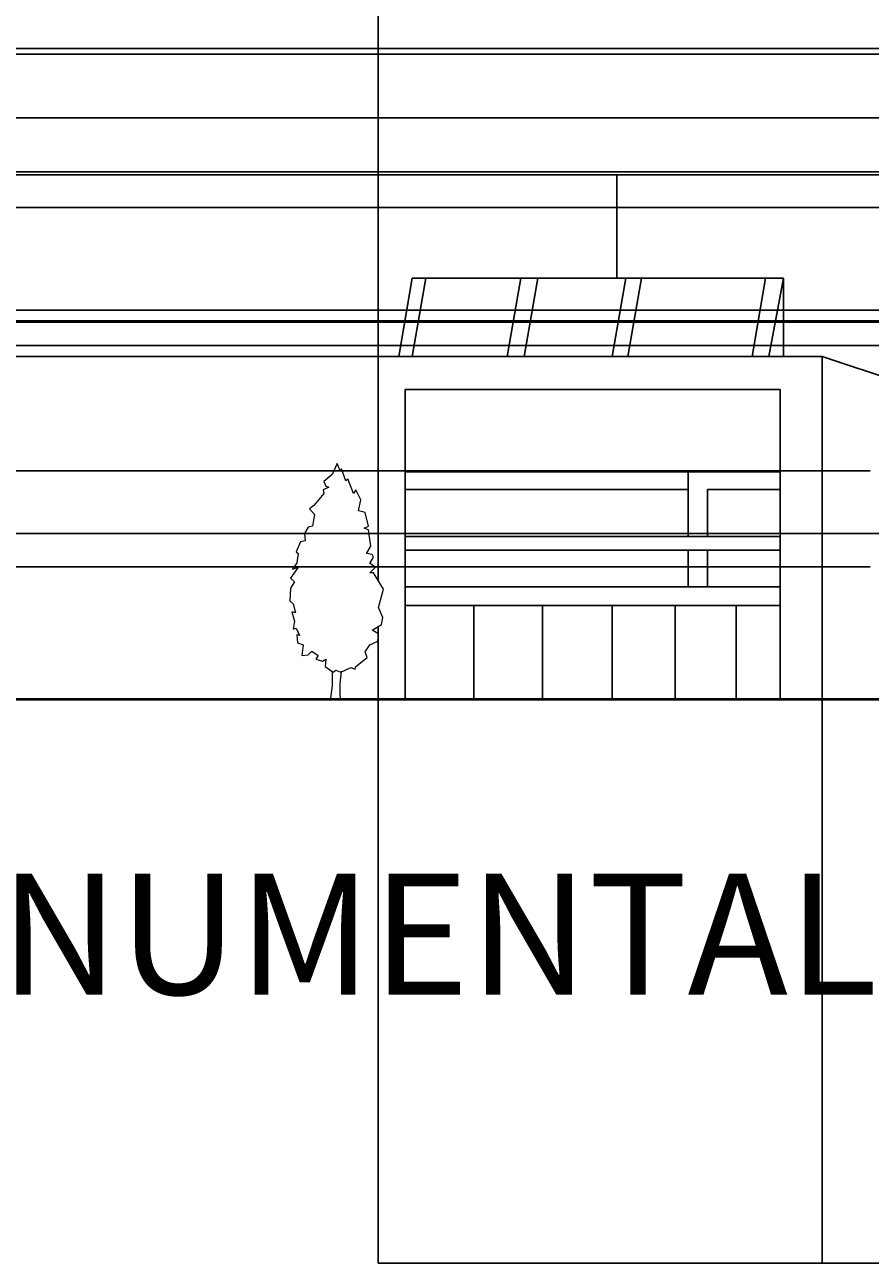
# Model space of a CAD drawing. Units: inches. Extents: x -32109 to 33221, y -19197 to 7608.
# Tile 8 of 25: x -20585 to -15627, y -5430 to 1836. Entities that reach past the tile are written whole.
import ezdxf

# ---------------------------------------------------------------- set-up
doc = ezdxf.new("R2010")
doc.units = ezdxf.units.IN
doc.header["$MEASUREMENT"] = 0
for name, color, linetype, lineweight in [('A-ANNO-DIMS', 2, 'Continuous', 18), ('A-ANNO-TEXT', 7, 'Continuous', 25), ('A-ELEV', 7, 'Continuous', 25), ('L-PLNT', 3, 'Continuous', 13)]:
    doc.layers.add(name, color=color, linetype=linetype, lineweight=lineweight)
doc.styles.get("Standard").update_dxf_attribs({"font": 'arial.ttf'})
doc.dimstyles.get("Standard").update_dxf_attribs({"dimtxt": 0.18, "dimasz": 0.18, "dimexe": 0.18, "dimexo": 0.0625, "dimgap": 0.09, "dimtad": 0, "dimtih": 1, "dimtoh": 1, "dimdec": 4, "dimzin": 0, "dimdsep": 46, "dimtxsty": 'Standard', "dimcen": 0.09, "dimadec": 0, "dimazin": 0, "dimtfac": 1, "dimtdec": 4, "dimtofl": 0, "dimtmove": 0, "dimatfit": 3, "dimfxl": 1, "dimtolj": 1, "dimtzin": 0, "dimarcsym": 0})

# ---------------------------------------------------------------- blocks, each defined once
blk = doc.blocks.new('*U2')
blk.add_lwpolyline([(-2.75400000000036, 191.699), (-6.7800000000002, 182.8509999999996), (-13.68200000000024, 176.9529999999995), (-11.95600000000013, 173.2659999999996), (-9.655999999999949, 172.529), (-14.25700000000006, 170.317), (-13.68200000000024, 167.3679999999999), (-21.73300000000017, 157.7829999999999), (-25.1840000000002, 154.8340000000003), (-21.15800000000036, 150.4099999999998), (-21.73300000000017, 147.4609999999998), (-22.88400000000001, 140.8249999999998), (-26.33400000000029, 140.087), (-29.21000000000004, 134.9259999999995), (-28.63499999999977, 129.0279999999998), (-32.66100000000006, 128.2909999999997), (-36.11099999999988, 120.1799999999998), (-34.38599999999997, 118.7059999999997), (-35.53600000000006, 111.3329999999996), (-38.98700000000008, 106.1709999999998), (-34.38599999999997, 107.6459999999997), (-40.71199999999999, 98.79799999999977), (-37.26099999999997, 95.8489999999997), (-40.71199999999999, 90.68799999999965), (-41.28700000000026, 80.36599999999999), (-38.41200000000026, 78.154), (-36.68600000000015, 70.78099999999995), (-39.5619999999999, 71.51799999999957), (-37.26099999999997, 64.14499999999998), (-38.41200000000026, 57.50899999999956), (-36.11099999999988, 58.24699999999984), (-33.23599999999988, 52.3479999999995), (-35.53600000000006, 53.08599999999978), (-34.96100000000024, 46.44999999999981), (-30.36000000000013, 44.9749999999999), (-31.50999999999977, 36.1279999999997), (-26.33400000000029, 36.86499999999978), (-23.45900000000029, 39.81399999999985), (-18.28300000000036, 36.1279999999997), (-20.00800000000027, 33.17799999999988), (-14.83199999999988, 31.70399999999972), (-11.95600000000013, 33.17799999999988), (-12.53099999999995, 27.27999999999975), (-6.204999999999927, 22.85599999999977), (-3.9050000000002, 24.33099999999968), (0.1209999999996398, 22.85599999999977), (8.172999999999774, 26.54299999999967), (11.62399999999979, 25.06799999999976), (12.19900000000007, 27.27999999999975), (21.40000000000009, 34.6529999999998), (19.67500000000018, 39.07699999999977), (23.70099999999957, 44.9749999999999), (30.02700000000004, 47.92399999999997), (30.60199999999986, 53.82299999999986), (25.42599999999993, 56.77199999999993), (32.90299999999979, 61.19599999999991), (34.05299999999988, 67.0939999999996), (30.60199999999986, 75.20499999999993), (34.6279999999997, 89.95100000000002), (26.57599999999957, 103.2219999999997), (23.70099999999957, 103.2219999999997), (28.30199999999968, 107.6459999999997), (23.70099999999957, 110.5949999999998), (26.57599999999957, 115.7559999999994), (25.42599999999993, 117.9679999999998), (20.82499999999982, 118.7059999999997), (24.27599999999984, 124.6040000000002), (22.55099999999993, 137.8759999999997), (19.09999999999991, 139.3499999999999), (22.55099999999993, 140.8249999999998), (19.67500000000018, 151.884), (14.49899999999979, 153.3589999999999), (16.22400000000016, 162.2069999999999), (12.19900000000007, 170.317), (10.47299999999995, 167.3679999999999), (5.871999999999843, 179.1649999999999), (4.146999999999934, 177.69), (0.6959999999999127, 187.2749999999996), (-0.4540000000001783, 185.7999999999997)], close=True)
for points in [[(-6.813000000000101, 23.66899999999987), (-6.813000000000101, 11.66899999999987), (-8.626999999999953, 0)], [(0.3869999999997162, 23.66899999999987), (-0.5760000000000219, 13.27099999999973), (-0.5760000000000219, 3.685999999999694), (0, 0)]]:
    blk.add_lwpolyline(points)
blk = doc.blocks.new('*D10')
at = {"layer": 'A-ANNO-DIMS', "color": 0, "lineweight": -2, "transparency": 16777216}
for p, q in [((-18512.646816, -110.179138), (-18512.646816, 5772.015489000001)), ((-18512.466816, 5771.835489), (-202.0927503703958, 5771.835489)), ((18109.136745, 5771.835489), (-201.2373206296045, 5771.835489)), ((18109.316745, -101.537382), (18109.316745, 5772.015489000001))]:
    blk.add_line(p, q, dxfattribs=at)
at = {"layer": 'A-ANNO-DIMS', "color": 0, "transparency": 16777216}
for points in [[(-18512.466816, 5771.865488999999), (-18512.466816, 5771.805489000001), (-18512.646816, 5771.835489)], [(18109.136745, 5771.865488999999), (18109.136745, 5771.805489000001), (18109.316745, 5771.835489)]]:
    blk.add_solid(points, dxfattribs=at)
at = {"layer": 'Defpoints', "color": 0, "transparency": 16777216}
for p in [(18109.316745, 5771.835489), (-18512.646816, -110.241638), (18109.316745, -101.599882)]:
    blk.add_point(p, dxfattribs=at)
at = {"layer": 'A-ANNO-DIMS', "color": 0, "transparency": 16777216, "insert": (-201.6650355000002, 5771.835489), "char_height": 0.18, "attachment_point": 5}
blk.add_mtext('\\A1;36622', dxfattribs=at)
blk = doc.blocks.new('*D11')
at = {"layer": 'A-ANNO-DIMS', "color": 0, "lineweight": -2, "transparency": 16777216}
for p, q in [((14509.612941, 1705.161904000001), (25710.64858400003, 1705.161904000003)), ((25710.46858400003, 1704.981904000003), (25710.46858400003, -209.6323674706641)), ((25710.46858400003, -2124.610567999994), (25710.46858400003, -209.9962965293272)), ((-18512.58431600001, -2124.790568000001), (25710.64858400003, -2124.790567999994))]:
    blk.add_line(p, q, dxfattribs=at)
at = {"layer": 'A-ANNO-DIMS', "color": 0, "transparency": 16777216}
for points in [[(25710.43858400003, 1704.981904000003), (25710.49858400002, 1704.981904000003), (25710.46858400003, 1705.161904000003)], [(25710.43858400003, -2124.610567999994), (25710.49858400002, -2124.610567999994), (25710.46858400003, -2124.790567999994)]]:
    blk.add_solid(points, dxfattribs=at)
at = {"layer": 'Defpoints', "color": 0, "transparency": 16777216}
for p in [(14509.550441, 1705.161904000001), (-18512.64681600001, -2124.790568000001), (25710.46858400003, -2124.790567999994)]:
    blk.add_point(p, dxfattribs=at)
at = {"layer": 'A-ANNO-DIMS', "color": 0, "transparency": 16777216, "insert": (25710.46858400002, -209.8143320000029), "char_height": 0.18, "attachment_point": 5}
blk.add_mtext('\\A1;3830', dxfattribs=at)
blk = doc.blocks.new('*D21')
at = {"layer": 'A-ANNO-DIMS', "color": 0, "lineweight": -2, "transparency": 16777216}
for p, q in [((-5532.163600000002, -1149.229573), (-24361.99565300002, -1149.229573000003)), ((-24361.81565300002, -1149.409573000004), (-24361.81565300002, -1636.828167362214)), ((-24361.81565300002, -2124.610568000004), (-24361.81565300002, -1637.191973637794)), ((-5677.141660000002, -2124.790568000001), (-24361.99565300002, -2124.790568000003))]:
    blk.add_line(p, q, dxfattribs=at)
at = {"layer": 'A-ANNO-DIMS', "color": 0, "transparency": 16777216}
for points in [[(-24361.84565300001, -1149.409573000004), (-24361.78565300002, -1149.409573000004), (-24361.81565300002, -1149.229573000003)], [(-24361.84565300001, -2124.610568000004), (-24361.78565300002, -2124.610568000004), (-24361.81565300002, -2124.790568000003)]]:
    blk.add_solid(points, dxfattribs=at)
at = {"layer": 'Defpoints', "color": 0, "transparency": 16777216}
for p in [(-24361.81565300002, -1149.229573000003), (-5532.101100000001, -1149.229573), (-5677.079160000002, -2124.790568000001)]:
    blk.add_point(p, dxfattribs=at)
at = {"layer": 'A-ANNO-DIMS', "color": 0, "transparency": 16777216, "insert": (-24361.81565300001, -1637.010070499996), "char_height": 0.18, "attachment_point": 5}
blk.add_mtext('\\A1;975.6', dxfattribs=at)
blk = doc.blocks.new('*D24')
at = {"layer": 'A-ANNO-DIMS', "color": 0, "lineweight": -2, "transparency": 16777216}
for p, q in [((-18512.646816, -2124.853068), (-18512.646816, -5429.734913)), ((-15909.074234, -2124.853068), (-15909.074234, -5429.734913)), ((-18512.466816, -5429.554913), (-17211.32562731923, -5429.554913)), ((-15909.254234, -5429.554913), (-17210.39542268076, -5429.554913))]:
    blk.add_line(p, q, dxfattribs=at)
at = {"layer": 'A-ANNO-DIMS', "color": 0, "transparency": 16777216}
for points in [[(-18512.466816, -5429.524913), (-18512.466816, -5429.584913), (-18512.646816, -5429.554913)], [(-15909.254234, -5429.524913), (-15909.254234, -5429.584913), (-15909.074234, -5429.554913)]]:
    blk.add_solid(points, dxfattribs=at)
at = {"layer": 'Defpoints', "color": 0, "transparency": 16777216}
for p in [(-18512.646816, -2124.790568), (-15909.074234, -2124.790568), (-15909.074234, -5429.554913)]:
    blk.add_point(p, dxfattribs=at)
at = {"layer": 'A-ANNO-DIMS', "color": 0, "transparency": 16777216, "insert": (-17210.860525, -5429.554913), "char_height": 0.18, "attachment_point": 5}
blk.add_mtext('\\A1;2603.6', dxfattribs=at)
blk = doc.blocks.new('*D25')
at = {"layer": 'A-ANNO-DIMS', "color": 0, "lineweight": -2, "transparency": 16777216}
for p, q in [((-15909.074234, -2124.853068), (-15909.074234, -5429.734913)), ((-15192.599186, -2124.853068), (-15192.599186, -5429.734913)), ((-15908.894234, -5429.554913), (-15551.2303525648, -5429.554913)), ((-15192.779186, -5429.554913), (-15550.4430674352, -5429.554913))]:
    blk.add_line(p, q, dxfattribs=at)
at = {"layer": 'A-ANNO-DIMS', "color": 0, "transparency": 16777216}
for points in [[(-15908.894234, -5429.524913), (-15908.894234, -5429.584913), (-15909.074234, -5429.554913)], [(-15192.779186, -5429.524913), (-15192.779186, -5429.584913), (-15192.599186, -5429.554913)]]:
    blk.add_solid(points, dxfattribs=at)
at = {"layer": 'Defpoints', "color": 0, "transparency": 16777216}
for p in [(-15909.074234, -2124.790568), (-15192.599186, -2124.790568), (-15192.599186, -5429.554913)]:
    blk.add_point(p, dxfattribs=at)
at = {"layer": 'A-ANNO-DIMS', "color": 0, "transparency": 16777216, "insert": (-15550.83671, -5429.554913), "char_height": 0.18, "attachment_point": 5}
blk.add_mtext('\\A1;716.5', dxfattribs=at)
blk = doc.blocks.new('*D35')
at = {"layer": 'A-ANNO-DIMS', "color": 0, "lineweight": -2, "transparency": 16777216}
for p, q in [((-18512.70931600001, -110.241638), (-24361.99565300002, -110.241638000001)), ((-24361.81565300002, -110.421638000001), (-24361.81565300002, -1117.334199862211)), ((-24361.81565300002, -2124.610568000002), (-24361.81565300002, -1117.698006137791)), ((-18512.70931600001, -2124.790568000001), (-24361.99565300002, -2124.790568000002))]:
    blk.add_line(p, q, dxfattribs=at)
at = {"layer": 'A-ANNO-DIMS', "color": 0, "transparency": 16777216}
for points in [[(-24361.84565300001, -110.421638000001), (-24361.78565300002, -110.421638000001), (-24361.81565300002, -110.241638000001)], [(-24361.84565300001, -2124.610568000002), (-24361.78565300002, -2124.610568000002), (-24361.81565300002, -2124.790568000002)]]:
    blk.add_solid(points, dxfattribs=at)
at = {"layer": 'Defpoints', "color": 0, "transparency": 16777216}
for p in [(-18512.64681600001, -110.241638), (-24361.81565300002, -2124.790568000002), (-18512.64681600001, -2124.790568000001)]:
    blk.add_point(p, dxfattribs=at)
at = {"layer": 'A-ANNO-DIMS', "color": 0, "transparency": 16777216, "insert": (-24361.81565300001, -1117.516102999994), "char_height": 0.18, "attachment_point": 5}
blk.add_mtext('\\A1;2014.5', dxfattribs=at)
blk = doc.blocks.new('*D36')
at = {"layer": 'A-ANNO-DIMS', "color": 0, "lineweight": -2, "transparency": 16777216}
for p, q in [((-17113.21748400001, 955.0880220000005), (-24361.99565300002, 955.0880219999992)), ((-24361.81565300002, 954.9080219999993), (-24361.81565300002, 422.6051565293307)), ((-24361.81565300002, -110.061638000001), (-24361.81565300002, 422.2412274706676)), ((-18512.70931600001, -110.241638), (-24361.99565300002, -110.241638000001))]:
    blk.add_line(p, q, dxfattribs=at)
at = {"layer": 'A-ANNO-DIMS', "color": 0, "transparency": 16777216}
for points in [[(-24361.84565300001, 954.9080219999993), (-24361.78565300002, 954.9080219999993), (-24361.81565300002, 955.0880219999992)], [(-24361.84565300001, -110.061638000001), (-24361.78565300002, -110.061638000001), (-24361.81565300002, -110.241638000001)]]:
    blk.add_solid(points, dxfattribs=at)
at = {"layer": 'Defpoints', "color": 0, "transparency": 16777216}
for p in [(-17113.15498400001, 955.0880220000005), (-24361.81565300002, -110.241638000001), (-18512.64681600001, -110.241638)]:
    blk.add_point(p, dxfattribs=at)
at = {"layer": 'A-ANNO-DIMS', "color": 0, "transparency": 16777216, "insert": (-24361.81565300001, 422.4231920000059), "char_height": 0.18, "attachment_point": 5}
blk.add_mtext('\\A1;1065.3', dxfattribs=at)
blk = doc.blocks.new('*D37')
at = {"layer": 'A-ANNO-DIMS', "color": 0, "lineweight": -2, "transparency": 16777216}
for p, q in [((-14538.09127400001, 1696.520148000001), (-24361.99565300002, 1696.520147999999)), ((-24361.81565300002, 1696.340147999999), (-24361.81565300002, -213.9532454706702)), ((-24361.81565300002, -2124.610568000003), (-24361.81565300002, -214.3171745293332)), ((-15192.66168600001, -2124.790568000001), (-24361.99565300002, -2124.790568000003))]:
    blk.add_line(p, q, dxfattribs=at)
at = {"layer": 'A-ANNO-DIMS', "color": 0, "transparency": 16777216}
for points in [[(-24361.84565300001, 1696.340147999999), (-24361.78565300002, 1696.340147999999), (-24361.81565300002, 1696.520147999999)], [(-24361.84565300001, -2124.610568000003), (-24361.78565300002, -2124.610568000003), (-24361.81565300002, -2124.790568000003)]]:
    blk.add_solid(points, dxfattribs=at)
at = {"layer": 'Defpoints', "color": 0, "transparency": 16777216}
for p in [(-14538.02877400001, 1696.520148000001), (-24361.81565300002, -2124.790568000003), (-15192.599186, -2124.790568000001)]:
    blk.add_point(p, dxfattribs=at)
at = {"layer": 'A-ANNO-DIMS', "color": 0, "transparency": 16777216, "insert": (-24361.81565300001, -214.1352099999948), "char_height": 0.18, "attachment_point": 5}
blk.add_mtext('\\A1;3821', dxfattribs=at)
blk = doc.blocks.new('*D38')
at = {"layer": 'A-ANNO-DIMS', "color": 0, "lineweight": -2, "transparency": 16777216}
for p, q in [((-11787.074272, -45.54407500000001), (-24361.99565300002, -45.54407500000204)), ((-24361.81565300002, -45.72407500000204), (-24361.81565300002, -1084.985418362212)), ((-24361.81565300002, -2124.610568000003), (-24361.81565300002, -1085.349224637792)), ((-11787.074272, -2124.790568000001), (-24361.99565300002, -2124.790568000003))]:
    blk.add_line(p, q, dxfattribs=at)
at = {"layer": 'A-ANNO-DIMS', "color": 0, "transparency": 16777216}
for points in [[(-24361.84565300001, -45.72407500000204), (-24361.78565300002, -45.72407500000204), (-24361.81565300002, -45.54407500000204)], [(-24361.84565300001, -2124.610568000003), (-24361.78565300002, -2124.610568000003), (-24361.81565300002, -2124.790568000003)]]:
    blk.add_solid(points, dxfattribs=at)
at = {"layer": 'Defpoints', "color": 0, "transparency": 16777216}
for p in [(-11787.011772, -45.54407500000001), (-24361.81565300002, -2124.790568000003), (-11787.011772, -2124.790568000001)]:
    blk.add_point(p, dxfattribs=at)
at = {"layer": 'A-ANNO-DIMS', "color": 0, "transparency": 16777216, "insert": (-24361.81565300001, -1085.167321499995), "char_height": 0.18, "attachment_point": 5}
blk.add_mtext('\\A1;2079.2', dxfattribs=at)
blk = doc.blocks.new('*D39')
at = {"layer": 'A-ANNO-DIMS', "color": 0, "lineweight": -2, "transparency": 16777216}
for p, q in [((-7375.940118000004, 1290.029218), (-24361.99565300002, 1290.029217999997)), ((-24361.81565300002, 1289.849217999998), (-24361.81565300002, -414.0189259706716)), ((-24361.81565300002, -2118.250999000004), (-24361.81565300002, -414.3828550293346)), ((-7754.474858000003, -2118.430999000001), (-24361.99565300002, -2118.430999000004))]:
    blk.add_line(p, q, dxfattribs=at)
at = {"layer": 'A-ANNO-DIMS', "color": 0, "transparency": 16777216}
for points in [[(-24361.84565300001, 1289.849217999998), (-24361.78565300002, 1289.849217999998), (-24361.81565300002, 1290.029217999997)], [(-24361.84565300001, -2118.250999000004), (-24361.78565300002, -2118.250999000004), (-24361.81565300002, -2118.430999000004)]]:
    blk.add_solid(points, dxfattribs=at)
at = {"layer": 'Defpoints', "color": 0, "transparency": 16777216}
for p in [(-7375.877618000004, 1290.029218), (-24361.81565300002, -2118.430999000004), (-7754.412358000003, -2118.430999000001)]:
    blk.add_point(p, dxfattribs=at)
at = {"layer": 'A-ANNO-DIMS', "color": 0, "transparency": 16777216, "insert": (-24361.81565300001, -414.2008904999961), "char_height": 0.18, "attachment_point": 5}
blk.add_mtext('\\A1;3408.5', dxfattribs=at)
blk = doc.blocks.new('*D40')
at = {"layer": 'A-ANNO-DIMS', "color": 0, "lineweight": -2, "transparency": 16777216}
for p, q in [((-5445.086779000002, 973.0114150000005), (-24361.99565300002, 973.0114149999976)), ((-24361.81565300002, 972.8314149999974), (-24361.81565300002, -575.7076119706716)), ((-24361.81565300002, -2124.610568000004), (-24361.81565300002, -576.0715410293345)), ((-5677.141660000002, -2124.790568000001), (-24361.99565300002, -2124.790568000003))]:
    blk.add_line(p, q, dxfattribs=at)
at = {"layer": 'A-ANNO-DIMS', "color": 0, "transparency": 16777216}
for points in [[(-24361.84565300001, 972.8314149999974), (-24361.78565300002, 972.8314149999974), (-24361.81565300002, 973.0114149999976)], [(-24361.84565300001, -2124.610568000004), (-24361.78565300002, -2124.610568000004), (-24361.81565300002, -2124.790568000003)]]:
    blk.add_solid(points, dxfattribs=at)
at = {"layer": 'Defpoints', "color": 0, "transparency": 16777216}
for p in [(-5445.024279000001, 973.0114150000005), (-24361.81565300002, -2124.790568000003), (-5677.079160000002, -2124.790568000001)]:
    blk.add_point(p, dxfattribs=at)
at = {"layer": 'A-ANNO-DIMS', "color": 0, "transparency": 16777216, "insert": (-24361.81565300001, -575.889576499996), "char_height": 0.18, "attachment_point": 5}
blk.add_mtext('\\A1;3098', dxfattribs=at)
blk = doc.blocks.new('*D41')
at = {"layer": 'A-ANNO-DIMS', "color": 0, "lineweight": -2, "transparency": 16777216}
for p, q in [((-651.0217760000003, 162.185712), (-24361.99565300002, 162.1857119999962)), ((-24361.81565300002, 162.0057119999962), (-24361.81565300002, -981.1205248622146)), ((-24361.81565300002, -2124.610568000005), (-24361.81565300002, -981.4843311377945)), ((-651.0217760000003, -2124.790568000001), (-24361.99565300002, -2124.790568000005))]:
    blk.add_line(p, q, dxfattribs=at)
at = {"layer": 'A-ANNO-DIMS', "color": 0, "transparency": 16777216}
for points in [[(-24361.84565300001, 162.0057119999962), (-24361.78565300002, 162.0057119999962), (-24361.81565300002, 162.1857119999962)], [(-24361.84565300001, -2124.610568000005), (-24361.78565300002, -2124.610568000005), (-24361.81565300002, -2124.790568000005)]]:
    blk.add_solid(points, dxfattribs=at)
at = {"layer": 'Defpoints', "color": 0, "transparency": 16777216}
for p in [(-650.9592760000002, 162.185712), (-24361.81565300002, -2124.790568000005), (-650.9592760000002, -2124.790568000001)]:
    blk.add_point(p, dxfattribs=at)
at = {"layer": 'A-ANNO-DIMS', "color": 0, "transparency": 16777216, "insert": (-24361.81565300001, -981.3024279999973), "char_height": 0.18, "attachment_point": 5}
blk.add_mtext('\\A1;2287', dxfattribs=at)
blk = doc.blocks.new('*D42')
at = {"layer": 'A-ANNO-DIMS', "color": 0, "lineweight": -2, "transparency": 16777216}
for p, q in [((-12501.42121900001, 764.1865930000002), (-24361.99565300002, 764.1865929999982)), ((-24361.81565300002, 764.0065929999982), (-24361.81565300002, 428.0747211377882)), ((-24361.81565300002, 91.77904299999811), (-24361.81565300002, 427.7109148622083)), ((-12488.224911, 91.59904300000002), (-24361.99565300002, 91.5990429999981))]:
    blk.add_line(p, q, dxfattribs=at)
at = {"layer": 'A-ANNO-DIMS', "color": 0, "transparency": 16777216}
for points in [[(-24361.84565300001, 764.0065929999982), (-24361.78565300002, 764.0065929999982), (-24361.81565300002, 764.1865929999982)], [(-24361.84565300001, 91.77904299999811), (-24361.78565300002, 91.77904299999811), (-24361.81565300002, 91.5990429999981)]]:
    blk.add_solid(points, dxfattribs=at)
at = {"layer": 'Defpoints', "color": 0, "transparency": 16777216}
for p in [(-12501.35871900001, 764.1865930000002), (-24361.81565300002, 91.5990429999981), (-12488.16241100001, 91.59904300000002)]:
    blk.add_point(p, dxfattribs=at)
at = {"layer": 'A-ANNO-DIMS', "color": 0, "transparency": 16777216, "insert": (-24361.81565300001, 427.892818000005), "char_height": 0.18, "attachment_point": 5}
blk.add_mtext('\\A1;672.6', dxfattribs=at)
blk = doc.blocks.new('*D43')
at = {"layer": 'A-ANNO-DIMS', "color": 0, "lineweight": -2, "transparency": 16777216}
for p, q in [((-7375.940118000004, 99.10345500000005), (-24361.99565300002, 99.10345499999731)), ((-24361.81565300002, 98.9234549999973), (-24361.81565300002, -1009.481868862213)), ((-24361.81565300002, -2118.250999000004), (-24361.81565300002, -1009.845675137793)), ((-7754.474858000003, -2118.430999000001), (-24361.99565300002, -2118.430999000004))]:
    blk.add_line(p, q, dxfattribs=at)
at = {"layer": 'A-ANNO-DIMS', "color": 0, "transparency": 16777216}
for points in [[(-24361.84565300001, 98.9234549999973), (-24361.78565300002, 98.9234549999973), (-24361.81565300002, 99.10345499999731)], [(-24361.84565300001, -2118.250999000004), (-24361.78565300002, -2118.250999000004), (-24361.81565300002, -2118.430999000004)]]:
    blk.add_solid(points, dxfattribs=at)
at = {"layer": 'Defpoints', "color": 0, "transparency": 16777216}
for p in [(-7375.877618000004, 99.10345500000005), (-24361.81565300002, -2118.430999000004), (-7754.412358000003, -2118.430999000001)]:
    blk.add_point(p, dxfattribs=at)
at = {"layer": 'A-ANNO-DIMS', "color": 0, "transparency": 16777216, "insert": (-24361.81565300001, -1009.663771999996), "char_height": 0.18, "attachment_point": 5}
blk.add_mtext('\\A1;2217.5', dxfattribs=at)
blk = doc.blocks.new('*D46')
at = {"layer": 'A-ANNO-DIMS', "color": 0, "lineweight": -2, "transparency": 16777216}
for p, q in [((-15626.56260400001, -780.5276970000004), (-24361.99565300002, -780.5276970000018)), ((-24361.81565300002, -780.7076970000016), (-24361.81565300002, -1062.24124897067)), ((-24361.81565300002, -1344.138730000002), (-24361.81565300002, -1062.605178029333)), ((-15626.56260400001, -1344.31873), (-24361.99565300002, -1344.318730000002))]:
    blk.add_line(p, q, dxfattribs=at)
at = {"layer": 'A-ANNO-DIMS', "color": 0, "transparency": 16777216}
for points in [[(-24361.84565300001, -780.7076970000016), (-24361.78565300002, -780.7076970000016), (-24361.81565300002, -780.5276970000018)], [(-24361.84565300001, -1344.138730000002), (-24361.78565300002, -1344.138730000002), (-24361.81565300002, -1344.318730000002)]]:
    blk.add_solid(points, dxfattribs=at)
at = {"layer": 'Defpoints', "color": 0, "transparency": 16777216}
for p in [(-15626.50010400001, -780.5276970000004), (-24361.81565300002, -1344.318730000002), (-15626.50010400001, -1344.31873)]:
    blk.add_point(p, dxfattribs=at)
at = {"layer": 'A-ANNO-DIMS', "color": 0, "transparency": 16777216, "insert": (-24361.81565300001, -1062.423213499994), "char_height": 0.18, "attachment_point": 5}
blk.add_mtext('\\A1;563.8', dxfattribs=at)
blk = doc.blocks.new('*D47')
at = {"layer": 'A-ANNO-DIMS', "color": 0, "lineweight": -2, "transparency": 16777216}
for p, q in [((-15626.56260400001, -1344.31873), (-24361.99565300002, -1344.318730000002)), ((-24361.81565300002, -1344.498730000002), (-24361.81565300002, -1734.372745862212)), ((-24361.81565300002, -2124.610568000003), (-24361.81565300002, -1734.736552137792)), ((-15909.136734, -2124.790568000001), (-24361.99565300002, -2124.790568000002))]:
    blk.add_line(p, q, dxfattribs=at)
at = {"layer": 'A-ANNO-DIMS', "color": 0, "transparency": 16777216}
for points in [[(-24361.84565300001, -1344.498730000002), (-24361.78565300002, -1344.498730000002), (-24361.81565300002, -1344.318730000002)], [(-24361.84565300001, -2124.610568000003), (-24361.78565300002, -2124.610568000003), (-24361.81565300002, -2124.790568000002)]]:
    blk.add_solid(points, dxfattribs=at)
at = {"layer": 'Defpoints', "color": 0, "transparency": 16777216}
for p in [(-15626.50010400001, -1344.31873), (-24361.81565300002, -2124.790568000002), (-15909.074234, -2124.790568000001)]:
    blk.add_point(p, dxfattribs=at)
at = {"layer": 'A-ANNO-DIMS', "color": 0, "transparency": 16777216, "insert": (-24361.81565300001, -1734.554648999995), "char_height": 0.18, "attachment_point": 5}
blk.add_mtext('\\A1;780.5', dxfattribs=at)
blk = doc.blocks.new('*D158')
at = {"layer": 'A-ANNO-DIMS', "color": 0, "lineweight": -2, "transparency": 16777216}
for p, q in [((5447.266114000002, 1662.169531000001), (-24361.99565300002, 1662.169530999996)), ((-24361.81565300002, 1661.989530999996), (-24361.81565300002, -230.1077594706735)), ((-24361.81565300002, -2122.568979000006), (-24361.81565300002, -230.4716885293365)), ((5279.201554000002, -2122.748979000001), (-24361.99565300002, -2122.748979000006))]:
    blk.add_line(p, q, dxfattribs=at)
at = {"layer": 'A-ANNO-DIMS', "color": 0, "transparency": 16777216}
for points in [[(-24361.84565300001, 1661.989530999996), (-24361.78565300002, 1661.989530999996), (-24361.81565300002, 1662.169530999996)], [(-24361.84565300001, -2122.568979000006), (-24361.78565300002, -2122.568979000006), (-24361.81565300002, -2122.748979000006)]]:
    blk.add_solid(points, dxfattribs=at)
at = {"layer": 'Defpoints', "color": 0, "transparency": 16777216}
for p in [(5447.328614000002, 1662.169531000001), (-24361.81565300002, -2122.748979000006), (5279.264054000002, -2122.748979000001)]:
    blk.add_point(p, dxfattribs=at)
at = {"layer": 'A-ANNO-DIMS', "color": 0, "transparency": 16777216, "insert": (-24361.81565300001, -230.289723999998), "char_height": 0.18, "attachment_point": 5}
blk.add_mtext('\\A1;3784.9', dxfattribs=at)

msp = doc.modelspace()

# ---------------------------------------------------------------- linework, layer by layer
at = {"layer": 'A-ELEV'}
for p, q in [((-15450.80606197804, 955.0880217890953), (-17113.15498428035, 955.0880217890954)), ((-17113.15498428035, 955.0880217890954), (-17113.15498428035, 349.1619627786568)), ((-18391.84596555905, -110.241637869025), (-18312.09679701138, 349.1619627786568)), ((-18312.37824431093, -110.241637869025), (-18232.62907576326, 349.1619627786568)), ((-18312.09679701138, 349.1619627786568), (-16135.38154622097, 349.1619627786568)), ((-17755.79390292504, -110.241637869025), (-17676.04473437737, 349.1619627786568)), ((-17655.33722856125, -110.241637869025), (-17575.58806001358, 349.1619627786568)), ((-17139.47847665622, -110.241637869025), (-17059.72930810855, 349.1619627786568)), ((-17047.16688347011, -110.241637869025), (-16967.41771492244, 349.1619627786568)), ((-16319.5347357981, -110.241637869025), (-16239.78556725043, 349.1619627786568)), ((-16135.38154622097, 349.1619627786568), (-16222.12805341536, -110.241637869025)), ((-16135.38154622097, 349.1619627786568), (-16135.38154622097, -110.241637869025)), ((-17113.15498428035, -110.241637869025), (-18512.64681618521, -110.241637869025)), ((-18512.64681618521, -110.241637869025), (-18512.64681618521, -1423.549618320588)), ((-17113.15498428035, -110.241637869025), (-15909.07423393536, -110.241637869025)), ((-15909.07423393536, -110.241637869025), (-15909.07423393536, -2124.790568085176)), ((-15909.07423393536, -110.241637869025), (-15189.72559618458, -350.2207840895844)), ((-18354.6766707229, -2124.790568085176), (-18354.6766707229, -303.6241125538509)), ((-18354.6766707229, -303.6241125538509), (-16155.29453934109, -303.6241125538509)), ((-16155.29453934109, -303.6241125538509), (-18354.6766707229, -303.6241125538509)), ((-16155.29453934109, -303.6241125538509), (-16155.29453934109, -2124.790568085176)), ((-16155.29453934109, -786.425186850116), (-18354.6766707229, -786.425186850116)), ((-16694.24849313559, -786.425186850116), (-16694.24849313559, -1167.328519107686)), ((-16694.24849313559, -889.8804440923267), (-18354.6766707229, -889.8804440923267)), ((-16155.29453934109, -889.8804440923267), (-16581.25300192991, -889.8804440923267)), ((-16581.2530019299, -889.8804440923267), (-16581.2530019299, -1167.328519107686)), ((-16155.29453934109, -1167.328519107686), (-18354.6766707229, -1167.328519107686)), ((-16155.29453934109, -1247.2711859798), (-18354.6766707229, -1247.2711859798)), ((-16694.24849313559, -1247.2711859798), (-16694.24849313559, -1461.144437094874)), ((-16581.2530019299, -1247.2711859798), (-16581.2530019299, -1461.144437094874)), ((-16694.24849313559, -1461.144437094874), (-18354.6766707229, -1461.144437094874)), ((-16694.24849313559, -1461.144437094874), (-16581.2530019299, -1461.144437094874)), ((-16155.29453934109, -1461.144437094874), (-16581.2530019299, -1461.144437094874)), ((-16155.29453934109, -1571.744371542241), (-18354.6766707229, -1571.744371542241)), ((-17952.1950988271, -2124.790568085177), (-17952.1950988271, -1571.744371542241)), ((-17549.3463419351, -2124.790568085177), (-17549.3463419351, -1571.744371542241)), ((-17139.89357929438, -2124.790568085177), (-17139.89357929438, -1571.744371542241)), ((-16770.065218331, -2124.790568085177), (-16770.065218331, -1571.744371542241)), ((-16413.44505245753, -2124.790568085177), (-16413.44505245753, -1571.744371542241)), ((-18512.64681618521, -1694.766471335513), (-18512.64681618521, -2124.790568085176)), ((-18512.64681618521, -2124.790568085177), (-21911.81565297427, -2124.790568085177)), ((-18512.64681618521, -2124.790568085177), (1683.58803657419, -2124.790568085177))]:
    msp.add_line(p, q, dxfattribs=at)

# ---------------------------------------------------------------- block references
at = {"layer": 'L-PLNT', "xscale": 7.247071498988421, "yscale": 7.247071498988421, "zscale": 7.247071498988421}
msp.add_blockref('*U2', (-18732.24619617269, -2127.10446931088), dxfattribs=at)

# ---------------------------------------------------------------- texts
at = {"layer": 'A-ANNO-TEXT'}
msp.add_text('MONUMENTAL    FRONT   FACADE    ( CONCEPTUAL ONLY   NO DIMENSIONS )', height=709.7949465747753, dxfattribs=at).set_placement((-22238.10681632875, -3853.851877923695))

# ---------------------------------------------------------------- dimensions: what is measured, and where the dimension line sits
at = {"layer": 'A-ANNO-DIMS'}
for base, p1, p2, override, picture, middle in [((18109.316745, 5771.835489), (-18512.646816, -110.241638), (18109.316745, -101.599882), {"dimdec": 0, "dimlfac": 1, "dimrnd": 0, "dimzin": 0, "dimdsep": 46, "dimlunit": 2}, '*D10', (-201.6650355000002, 5771.835489)), ((-15909.074234, -5429.554913), (-18512.646816, -2124.790568), (-15909.074234, -2124.790568), {"dimdec": 1, "dimlfac": 1, "dimrnd": 0, "dimzin": 0, "dimdsep": 46, "dimlunit": 2}, '*D24', (-17210.860525, -5429.554913)), ((-15192.599186, -5429.554913), (-15909.074234, -2124.790568), (-15192.599186, -2124.790568), {"dimdec": 1, "dimlfac": 1, "dimrnd": 0, "dimzin": 0, "dimdsep": 46, "dimlunit": 2}, '*D25', (-15550.83671, -5429.554913))]:
    dim = msp.add_linear_dim(base=base, p1=p1, p2=p2, dimstyle='Standard', override=override, dxfattribs=at)
    dim.commit()
    dim.dimension.update_dxf_attribs({"geometry": picture, "text_midpoint": middle})
for base, p1, p2, override, picture, middle in [((-24361.81565300002, -2124.790568000003), (-14538.028774, 1696.520148), (-15192.599186, -2124.790568), {"dimdec": 0, "dimlfac": 1, "dimrnd": 0, "dimzin": 0, "dimdsep": 46, "dimlunit": 2}, '*D37', (-24361.81565300001, -214.1352099999948)), ((25710.46858400003, -2124.790567999994), (14509.550441, 1705.161904), (-18512.646816, -2124.790568), {"dimdec": 0, "dimlfac": 1, "dimrnd": 0, "dimzin": 0, "dimdsep": 46, "dimlunit": 2}, '*D11', (25710.46858400002, -209.8143320000029)), ((-24361.81565300002, -2122.748979000006), (5447.328613999999, 1662.169531), (5279.264054, -2122.748979), {"dimdec": 1, "dimlfac": 1, "dimrnd": 0, "dimzin": 0, "dimdsep": 46, "dimlunit": 2}, '*D158', (-24361.81565300001, -230.289723999998)), ((-24361.81565300002, -2118.430999000004), (-7375.877618000001, 1290.029218), (-7754.412358, -2118.430999), {"dimdec": 1, "dimlfac": 1, "dimrnd": 0, "dimzin": 0, "dimdsep": 46, "dimlunit": 2}, '*D39', (-24361.81565300001, -414.2008904999961)), ((-24361.81565300002, -110.241638000001), (-17113.154984, 955.0880219999999), (-18512.646816, -110.241638), {"dimdec": 1, "dimlfac": 1, "dimrnd": 0, "dimzin": 0, "dimdsep": 46, "dimlunit": 2}, '*D36', (-24361.81565300001, 422.4231920000059)), ((-24361.81565300002, -2124.790568000003), (-5445.024279, 973.011415), (-5677.07916, -2124.790568), {"dimdec": 0, "dimlfac": 1, "dimrnd": 0, "dimzin": 0, "dimdsep": 46, "dimlunit": 2}, '*D40', (-24361.81565300001, -575.889576499996)), ((-24361.81565300002, 91.5990429999981), (-12501.358719, 764.186593), (-12488.162411, 91.599043), {"dimdec": 1, "dimlfac": 1, "dimrnd": 0, "dimzin": 0, "dimdsep": 46, "dimlunit": 2}, '*D42', (-24361.81565300001, 427.892818000005)), ((-24361.81565300002, -2124.790568000005), (-650.959276, 162.185712), (-650.959276, -2124.790568), {"dimdec": 0, "dimlfac": 1, "dimrnd": 0, "dimzin": 0, "dimdsep": 46, "dimlunit": 2}, '*D41', (-24361.81565300001, -981.3024279999973)), ((-24361.81565300002, -2118.430999000004), (-7375.877618000001, 99.103455), (-7754.412358, -2118.430999), {"dimdec": 1, "dimlfac": 1, "dimrnd": 0, "dimzin": 0, "dimdsep": 46, "dimlunit": 2}, '*D43', (-24361.81565300001, -1009.663771999996)), ((-24361.81565300002, -2124.790568000003), (-11787.011772, -45.54407499999999), (-11787.011772, -2124.790568), {"dimdec": 1, "dimlfac": 1, "dimrnd": 0, "dimzin": 0, "dimdsep": 46, "dimlunit": 2}, '*D38', (-24361.81565300001, -1085.167321499995)), ((-24361.81565300002, -2124.790568000002), (-18512.646816, -110.241638), (-18512.646816, -2124.790568), {"dimdec": 1, "dimlfac": 1, "dimrnd": 0, "dimzin": 0, "dimdsep": 46, "dimlunit": 2}, '*D35', (-24361.81565300001, -1117.516102999994)), ((-24361.81565300002, -1344.318730000002), (-15626.500104, -780.527697), (-15626.500104, -1344.31873), {"dimdec": 1, "dimlfac": 1, "dimrnd": 0, "dimzin": 0, "dimdsep": 46, "dimlunit": 2}, '*D46', (-24361.81565300001, -1062.423213499994)), ((-24361.81565300002, -1149.229573000003), (-5677.07916, -2124.790568), (-5532.1011, -1149.229573), {"dimdec": 1, "dimlfac": 1, "dimrnd": 0, "dimzin": 0, "dimdsep": 46, "dimlunit": 2}, '*D21', (-24361.81565300001, -1637.010070499996)), ((-24361.81565300002, -2124.790568000002), (-15626.500104, -1344.31873), (-15909.074234, -2124.790568), {"dimdec": 1, "dimlfac": 1, "dimrnd": 0, "dimzin": 0, "dimdsep": 46, "dimlunit": 2}, '*D47', (-24361.81565300001, -1734.554648999995))]:
    dim = msp.add_linear_dim(base=base, p1=p1, p2=p2, angle=90, dimstyle='Standard', override=override, dxfattribs=at)
    dim.commit()
    dim.dimension.update_dxf_attribs({"geometry": picture, "text_midpoint": middle})

doc.saveas('drawing.dxf')
